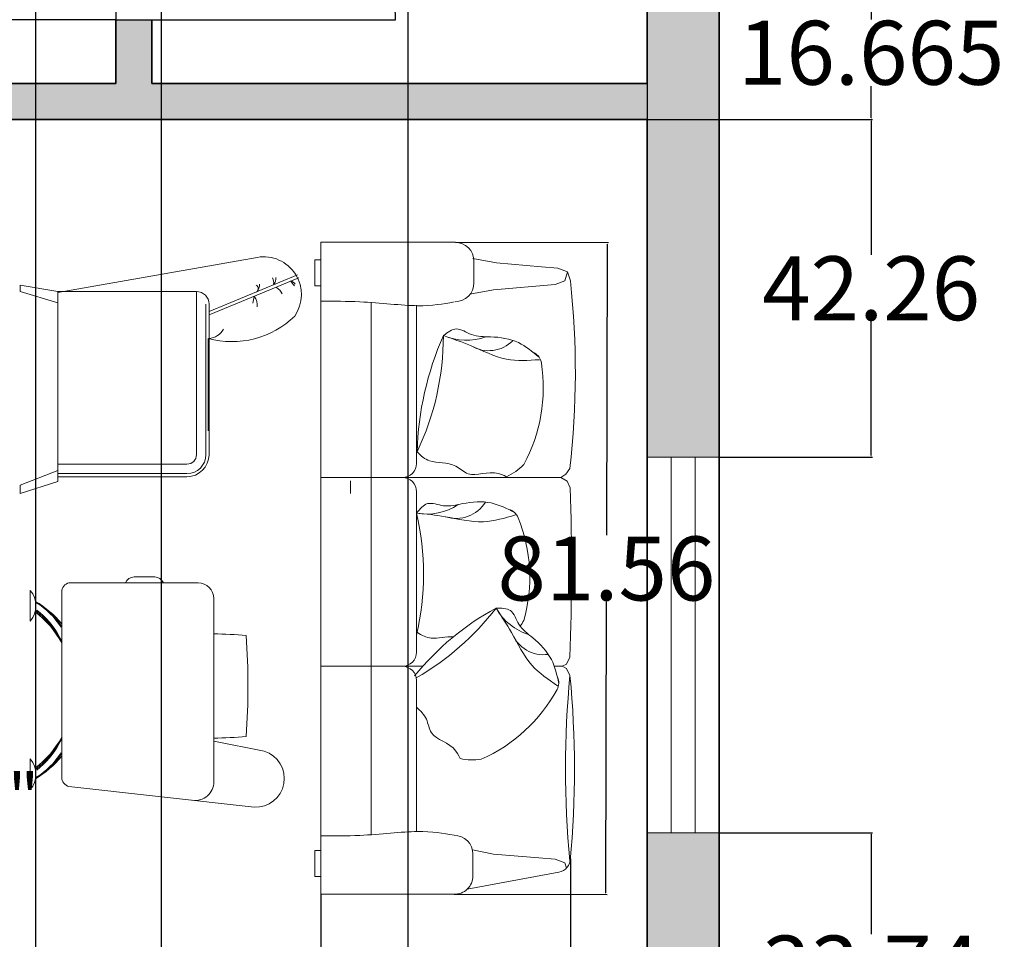
# Model space of a CAD drawing. Units: inches. Extents: x -24 to 368, y -370 to 58.
# Tile 6 of 9: x 235 to 358, y -255 to -140. Entities that reach past the tile are written whole.
import ezdxf

# ---------------------------------------------------------------- set-up
doc = ezdxf.new("R2010")
doc.units = ezdxf.units.IN
doc.header["$MEASUREMENT"] = 0
for name, color, linetype, lineweight in [('A-ANNO-DIMS', 2, 'Continuous', 18), ('A-AREA-IDEN', 7, 'Continuous', 18), ('A-WALL', 7, 'Continuous', 35), ('Furniture', 7, 'Continuous', 15)]:
    doc.layers.add(name, color=color, linetype=linetype, lineweight=lineweight)
for name, color, linetype, lineweight, true_color in [('A-DOOR', 40, 'Continuous', 25, 0xf8d731), ('A-GLAZ', 30, 'Continuous', 18, 0xf26722), ('A-WALL-PATT', 18, 'Continuous', 13, 0x000000)]:
    doc.layers.add(name, color=color, linetype=linetype, lineweight=lineweight, true_color=true_color)
doc.styles.get("Standard").update_dxf_attribs({"font": 'arial.ttf'})
doc.dimstyles.get("Standard").update_dxf_attribs({"dimtxt": 8, "dimasz": 0.18, "dimexe": 0.18, "dimexo": 0.0625, "dimgap": 0.09, "dimtad": 0, "dimtih": 1, "dimtoh": 1, "dimdec": 4, "dimzin": 0, "dimdsep": 46, "dimlunit": 3, "dimtxsty": 'Standard', "dimcen": 0.09, "dimclre": 5, "dimclrt": 6, "dimadec": 0, "dimazin": 0, "dimtfac": 1, "dimtdec": 4, "dimtofl": 0, "dimtmove": 0, "dimatfit": 3, "dimfxl": 1, "dimtolj": 1, "dimtzin": 0, "dimarcsym": 0})

# ---------------------------------------------------------------- blocks, each defined once
blk = doc.blocks.new('WINDOW-47-JAMB-DETAIL')
for p, q in [((0, 9), (47, 9)), ((0, 0), (0, 9)), ((0, 9), (0, 4.5)), ((47, 9), (47, 0)), ((0, 6), (47, 6)), ((0, 3), (47, 3)), ((47, 0), (0, 0))]:
    blk.add_line(p, q)
blk = doc.blocks.new('DOOR-SINGLE-35')
for p, q in [((0, 35), (0, 0)), ((0, 35), (4.5, 35)), ((0, 2), (35, 2)), ((0, 0), (35, 0)), ((0, 0), (4.5, 0))]:
    blk.add_line(p, q)
blk.add_arc((0, 0), 35, 0, 90)
blk = doc.blocks.new('*D34')
at = {"layer": 'A-ANNO-DIMS', "color": 5, "lineweight": -2, "transparency": 16777216}
for p, q in [((322.22, -241.61), (341.36, -241.61)), ((313.22, -275.36), (341.36, -275.36))]:
    blk.add_line(p, q, dxfattribs=at)
at = {"layer": 'A-ANNO-DIMS', "color": 0, "lineweight": -2, "transparency": 16777216}
for p, q in [((341.18, -241.79), (341.18, -254.31)), ((341.18, -275.18), (341.18, -262.66))]:
    blk.add_line(p, q, dxfattribs=at)
at = {"layer": 'A-ANNO-DIMS', "color": 0, "transparency": 16777216}
for points in [[(341.15, -241.79), (341.21, -241.79), (341.18, -241.61)], [(341.15, -275.18), (341.21, -275.18), (341.18, -275.36)]]:
    blk.add_solid(points, dxfattribs=at)
at = {"layer": 'Defpoints', "color": 0, "transparency": 16777216}
for p in [(322.16, -241.61), (341.18, -241.61), (313.16, -275.36)]:
    blk.add_point(p, dxfattribs=at)
at = {"layer": 'A-ANNO-DIMS', "color": 6, "transparency": 16777216, "insert": (341.18, -258.49), "char_height": 8, "attachment_point": 5}
blk.add_mtext('\\A1;33.74', dxfattribs=at)
blk = doc.blocks.new('*D35')
at = {"layer": 'A-ANNO-DIMS', "color": 5, "lineweight": -2, "transparency": 16777216}
for p, q in [((313.22, -152.36), (341.36, -152.36)), ((322.22, -194.61), (341.36, -194.61))]:
    blk.add_line(p, q, dxfattribs=at)
at = {"layer": 'A-ANNO-DIMS', "color": 0, "lineweight": -2, "transparency": 16777216}
for p, q in [((341.18, -152.54), (341.18, -169.31)), ((341.18, -194.43), (341.18, -177.66))]:
    blk.add_line(p, q, dxfattribs=at)
at = {"layer": 'A-ANNO-DIMS', "color": 0, "transparency": 16777216}
for points in [[(341.15, -152.54), (341.21, -152.54), (341.18, -152.36)], [(341.15, -194.43), (341.21, -194.43), (341.18, -194.61)]]:
    blk.add_solid(points, dxfattribs=at)
at = {"layer": 'Defpoints', "color": 0, "transparency": 16777216}
for p in [(313.16, -152.36), (341.18, -152.36), (322.16, -194.61)]:
    blk.add_point(p, dxfattribs=at)
at = {"layer": 'A-ANNO-DIMS', "color": 6, "transparency": 16777216, "insert": (341.18, -173.49), "char_height": 8, "attachment_point": 5}
blk.add_mtext('\\A1;42.26', dxfattribs=at)
blk = doc.blocks.new('*D36')
at = {"layer": 'A-ANNO-DIMS', "color": 5, "lineweight": -2, "transparency": 16777216}
for p, q in [((322.22, -135.69), (341.36, -135.69)), ((313.22, -152.36), (341.36, -152.36))]:
    blk.add_line(p, q, dxfattribs=at)
at = {"layer": 'A-ANNO-DIMS', "color": 0, "lineweight": -2, "transparency": 16777216}
for p, q in [((341.18, -135.87), (341.18, -139.85)), ((341.18, -152.18), (341.18, -148.2))]:
    blk.add_line(p, q, dxfattribs=at)
at = {"layer": 'A-ANNO-DIMS', "color": 0, "transparency": 16777216}
for points in [[(341.15, -135.87), (341.21, -135.87), (341.18, -135.69)], [(341.15, -152.18), (341.21, -152.18), (341.18, -152.36)]]:
    blk.add_solid(points, dxfattribs=at)
at = {"layer": 'Defpoints', "color": 0, "transparency": 16777216}
for p in [(322.16, -135.69), (341.18, -135.69), (313.16, -152.36)]:
    blk.add_point(p, dxfattribs=at)
at = {"layer": 'A-ANNO-DIMS', "color": 6, "transparency": 16777216, "insert": (341.18, -144.02), "char_height": 8, "attachment_point": 5}
blk.add_mtext('\\A1;16.665', dxfattribs=at)
blk = doc.blocks.new('*D43')
at = {"layer": 'A-ANNO-DIMS', "color": 5, "lineweight": -2, "transparency": 16777216}
for p, q in [((283.21, 24.58), (283.21, -363.55)), ((313.16, 24.58), (313.16, -363.55))]:
    blk.add_line(p, q, dxfattribs=at)
at = {"layer": 'A-ANNO-DIMS', "color": 0, "lineweight": -2, "transparency": 16777216}
for p, q in [((283.39, -363.37), (284.5, -363.37)), ((312.98, -363.37), (311.87, -363.37))]:
    blk.add_line(p, q, dxfattribs=at)
at = {"layer": 'A-ANNO-DIMS', "color": 0, "transparency": 16777216}
for points in [[(283.39, -363.34), (283.39, -363.4), (283.21, -363.37)], [(312.98, -363.34), (312.98, -363.4), (313.16, -363.37)]]:
    blk.add_solid(points, dxfattribs=at)
at = {"layer": 'Defpoints', "color": 0, "transparency": 16777216}
for p in [(283.21, 24.64), (313.16, 24.64), (313.16, -363.37)]:
    blk.add_point(p, dxfattribs=at)
at = {"layer": 'A-ANNO-DIMS', "color": 6, "transparency": 16777216, "insert": (298.19, -363.37), "char_height": 8, "attachment_point": 5}
blk.add_mtext('\\A1;29.95', dxfattribs=at)
blk = doc.blocks.new('*D59')
at = {"layer": 'A-ANNO-DIMS', "color": 5, "lineweight": -2, "transparency": 16777216}
for p, q in [((246.6, -139.91), (-15.03, -139.91)), ((246.6, -147.86), (-15.03, -147.86))]:
    blk.add_line(p, q, dxfattribs=at)
at = {"layer": 'A-ANNO-DIMS', "color": 0, "lineweight": -2, "transparency": 16777216}
for p, q in [((-14.85, -139.91), (-14.85, -139.73)), ((-14.85, -139.73), (-14.67, -139.73)), ((-14.85, -147.68), (-14.85, -140.09))]:
    blk.add_line(p, q, dxfattribs=at)
at = {"layer": 'A-ANNO-DIMS', "color": 0, "transparency": 16777216}
for points in [[(-14.88, -140.09), (-14.82, -140.09), (-14.85, -139.91)], [(-14.88, -147.68), (-14.82, -147.68), (-14.85, -147.86)]]:
    blk.add_solid(points, dxfattribs=at)
at = {"layer": 'Defpoints', "color": 0, "transparency": 16777216}
for p in [(-14.85, -139.91), (246.66, -139.91), (246.66, -147.86)]:
    blk.add_point(p, dxfattribs=at)
at = {"layer": 'A-ANNO-DIMS', "color": 6, "transparency": 16777216, "insert": (-4.2, -139.73), "char_height": 8, "attachment_point": 5}
blk.add_mtext('\\A1;7.95', dxfattribs=at)
blk = doc.blocks.new('*D61')
at = {"layer": 'A-ANNO-DIMS', "color": 5, "lineweight": -2, "transparency": 16777216}
for p, q in [((236.66, -275.29), (236.66, 52.85)), ((252.39, -275.29), (252.39, 52.85))]:
    blk.add_line(p, q, dxfattribs=at)
at = {"layer": 'A-ANNO-DIMS', "color": 0, "lineweight": -2, "transparency": 16777216}
for p, q in [((236.84, 52.67), (252.21, 52.67)), ((252.39, 52.67), (252.57, 52.67))]:
    blk.add_line(p, q, dxfattribs=at)
at = {"layer": 'A-ANNO-DIMS', "color": 0, "transparency": 16777216}
for points in [[(236.84, 52.7), (236.84, 52.64), (236.66, 52.67)], [(252.21, 52.7), (252.21, 52.64), (252.39, 52.67)]]:
    blk.add_solid(points, dxfattribs=at)
at = {"layer": 'Defpoints', "color": 0, "transparency": 16777216}
for p in [(252.39, 52.67), (236.66, -275.36), (252.39, -275.36)]:
    blk.add_point(p, dxfattribs=at)
at = {"layer": 'A-ANNO-DIMS', "color": 6, "transparency": 16777216, "insert": (265.78, 52.67), "char_height": 8, "attachment_point": 5}
blk.add_mtext('\\A1;15.73', dxfattribs=at)
blk = doc.blocks.new('*D66')
at = {"layer": 'A-ANNO-DIMS', "color": 5, "lineweight": -2, "transparency": 16777216}
for p, q in [((289.18, -167.74), (308.31, -167.77)), ((289.02, -249.3), (308.16, -249.33))]:
    blk.add_line(p, q, dxfattribs=at)
at = {"layer": 'A-ANNO-DIMS', "color": 0, "lineweight": -2, "transparency": 16777216}
for p, q in [((308.13, -167.95), (308.06, -204.38)), ((307.98, -249.15), (308.05, -212.73))]:
    blk.add_line(p, q, dxfattribs=at)
at = {"layer": 'A-ANNO-DIMS', "color": 0, "transparency": 16777216}
for points in [[(308.1, -167.95), (308.16, -167.95), (308.13, -167.77)], [(307.95, -249.15), (308.01, -249.15), (307.98, -249.33)]]:
    blk.add_solid(points, dxfattribs=at)
at = {"layer": 'Defpoints', "color": 0, "transparency": 16777216}
for p in [(289.11, -167.74), (288.96, -249.3), (307.98, -249.33)]:
    blk.add_point(p, dxfattribs=at)
at = {"layer": 'A-ANNO-DIMS', "color": 6, "transparency": 16777216, "insert": (308.05, -208.55), "char_height": 8, "attachment_point": 5}
blk.add_mtext('\\A1;81.56', dxfattribs=at)
blk = doc.blocks.new('*D67')
at = {"layer": 'A-ANNO-DIMS', "color": 5, "lineweight": -2, "transparency": 16777216}
for p, q in [((303.55, -244.87), (303.55, -363.55)), ((272.33, -249.36), (272.33, -363.55))]:
    blk.add_line(p, q, dxfattribs=at)
at = {"layer": 'A-ANNO-DIMS', "color": 0, "lineweight": -2, "transparency": 16777216}
for p, q in [((272.51, -363.37), (274.4, -363.37)), ((303.37, -363.37), (301.49, -363.37))]:
    blk.add_line(p, q, dxfattribs=at)
at = {"layer": 'A-ANNO-DIMS', "color": 0, "transparency": 16777216}
for points in [[(272.51, -363.34), (272.51, -363.4), (272.33, -363.37)], [(303.37, -363.34), (303.37, -363.4), (303.55, -363.37)]]:
    blk.add_solid(points, dxfattribs=at)
at = {"layer": 'Defpoints', "color": 0, "transparency": 16777216}
for p in [(303.55, -244.81), (272.33, -249.3), (303.55, -363.37)]:
    blk.add_point(p, dxfattribs=at)
at = {"layer": 'A-ANNO-DIMS', "color": 6, "transparency": 16777216, "insert": (287.94, -363.37), "char_height": 8, "attachment_point": 5}
blk.add_mtext('\\A1;31.22', dxfattribs=at)

msp = doc.modelspace()

# ---------------------------------------------------------------- hatches: boundary and pattern name
at = {"layer": 'A-WALL-PATT'}
h = msp.add_hatch(color=256, dxfattribs=at)
h.dxf.hatch_style = 1
h.paths.add_polyline_path([(13.1621, -93.8573), (80.4499, -93.8573), (80.4499, -89.3573), (13.1621, -89.3573), (13.1621, -61.0987), (4.1621, -61.0987), (4.1621, -149.8573), (13.1621, -149.8573)])
h.paths.add_polyline_path([(146.5668, -27.3573), (133.1621, -27.3573), (133.1621, 10.3323), (133.1272, 10.3313), (133.1621, 24.6427), (139.8141, 24.6427), (139.8141, 33.6427), (95.3329, 33.6427), (95.3329, 24.6427), (128.6621, 24.6427), (128.6621, -89.3573), (127.4499, -89.3573), (127.4499, -93.8573), (133.1621, -93.8573), (133.1621, -31.8573), (146.5668, -31.8573)])
h.paths.add_polyline_path([(197.6621, 24.6427), (236.2134, 24.6427), (236.2134, 33.6427), (169.8141, 33.6427), (169.8141, 24.6427), (193.1621, 24.6427), (193.1621, -27.3573), (181.5668, -27.3573), (181.5668, -31.8573), (193.1621, -31.8573), (193.1621, -95.8573), (199.2127, -95.8573), (199.2127, -91.3573), (197.6621, -91.3573)])
h.paths.add_polyline_path([(322.1621, -52.531), (313.1621, -52.531), (313.1621, -91.3573), (246.2127, -91.3573), (246.2127, -95.8573), (246.6621, -95.8573), (246.6621, -104.9077), (251.1621, -104.9077), (251.1621, -95.8573), (313.1621, -95.8573), (313.1621, -105.6922), (317.6621, -105.6922), (322.1621, -105.6922)])
h.paths.add_polyline_path([(322.1621, -135.6922), (313.1621, -135.6922), (313.1621, -147.8573), (251.1621, -147.8573), (251.1621, -139.9077), (246.6621, -139.9077), (246.6621, -147.8573), (199.43, -147.8573), (199.43, -152.3573), (313.1621, -152.3573), (313.1621, -194.6142), (317.6621, -194.6142), (322.1621, -194.6142)])
h.paths.add_polyline_path([(322.1621, -241.6142), (313.1621, -241.6142), (313.1621, -275.3573), (287.3912, -275.3573), (287.3912, -279.8573), (313.1621, -279.8573), (313.1621, -335.3573), (298.077, -335.3573), (298.077, -344.3573), (322.1621, -344.3573)])
h.paths.add_polyline_path([(263.077, -335.3573), (241.1621, -335.3573), (241.1621, -279.8573), (252.3912, -279.8573), (252.3912, -275.3573), (236.6621, -275.3573), (236.6621, -298.8573), (234.5689, -298.8573), (234.5689, -303.3573), (236.6621, -303.3573), (236.6621, -344.3573), (263.077, -344.3573), (263.077, -339.8573)])
h.paths.add_polyline_path([(175.5689, -298.8573), (131.6621, -298.8573), (131.6621, -152.3573), (164.43, -152.3573), (164.43, -147.8573), (127.1621, -147.8573), (127.1621, -232.8573), (117.1621, -232.8573), (117.1621, -237.3573), (127.1621, -237.3573), (127.1621, -335.3573), (84.4055, -335.3573), (84.4055, -344.3573), (131.6621, -344.3573), (131.6621, -303.3573), (175.5689, -303.3573)])
h.paths.add_polyline_path([(70.1621, -232.8573), (13.1621, -232.8573), (13.1621, -196.8573), (4.1621, -196.8573), (4.1621, -257.9061), (13.1621, -257.9061), (13.1621, -237.3573), (70.1621, -237.3573)])
h.paths.add_polyline_path([(13.1621, -304.9061), (4.1621, -304.9061), (4.1621, -344.3573), (37.4055, -344.3573), (37.4055, -335.3573), (13.1621, -335.3573)])
h.paths.add_polyline_path([(322.1621, 33.6427), (283.2134, 33.6427), (283.2134, 24.6427), (313.1621, 24.6427), (313.1621, 11.9273), (313.4656, 11.629), (313.1621, 11.629), (313.1621, -5.531), (322.1621, -5.531)])
h.paths.add_polyline_path([(48.3329, 33.6427), (4.1621, 33.6427), (4.1621, -14.0987), (13.1621, -14.0987), (13.1621, 24.6427), (48.3329, 24.6427)])

# ---------------------------------------------------------------- linework, layer by layer
at = {"layer": 'A-WALL'}
for p, q in [((322.1621, 33.6427), (322.1621, -344.3573)), ((313.1621, -95.8573), (313.1621, -147.8573)), ((246.6621, -139.9077), (246.6621, -147.8573)), ((251.1621, -139.9077), (251.1621, -147.8573)), ((199.43, -147.8573), (246.6621, -147.8573)), ((251.1621, -147.8573), (313.1621, -147.8573)), ((199.43, -152.3573), (313.1621, -152.3573)), ((313.1621, -152.3573), (313.1621, -232.8573)), ((313.1621, -232.8573), (313.1621, -275.3573))]:
    msp.add_line(p, q, dxfattribs=at)
at = {"layer": 'Furniture'}
for p, q in [((272.3319, -249.2987, 13.1343), (272.3323, -167.7325, -0.364)), ((289.1148, -167.7387, -0.364), (272.3323, -167.7325, -0.364)), ((264.3556, -169.6195), (239.4285, -174.032)), ((271.546, -169.9319), (271.546, -173.2035)), ((272.3323, -169.9319), (271.546, -169.9319)), ((291.3267, -169.7474, -0.364), (294.2813, -170.3225, -0.364)), ((291.4762, -170.1009, -0.364), (291.4762, -172.808, -0.364)), ((294.2813, -170.3225, -0.364), (299.9427, -170.8003, -0.364)), ((299.9427, -170.8003, -0.364), (301.9905, -170.9604, -0.364)), ((301.9905, -170.9604, -0.364), (303.1934, -171.4178, -0.364)), ((269.4035, -171.8269), (258.327, -176.3942)), ((269.5451, -172.1943), (258.327, -176.82)), ((302.8372, -172.5743, -0.364), (303.1934, -171.4178, -0.364)), ((303.1934, -171.4178, -0.364), (303.5496, -172.5743, -0.364)), ((234.705, -173.901), (234.705, -173.1136)), ((234.705, -173.1136), (239.4294, -173.901)), ((271.546, -173.2035), (272.3322, -173.2035, 0.5414)), ((290.9705, -174.2447, -0.364), (293.9251, -173.6696, -0.364)), ((293.9251, -173.6696, -0.364), (301.6343, -173.0317, -0.364)), ((301.6343, -173.0317, -0.364), (302.8372, -172.5743, -0.364)), ((239.4196, -175.2986), (234.705, -173.901)), ((239.4294, -173.901), (239.4196, -175.2986)), ((256.7522, -173.901), (239.4294, -173.901)), ((239.4294, -197.6823), (239.4294, -173.9994)), ((256.7522, -194.3143), (256.7522, -173.901)), ((257.9333, -179.7879), (257.9333, -175.4758)), ((258.327, -179.7879), (258.327, -175.4758)), ((278.5971, -175.267, 9.5261), (278.5971, -241.8677, 9.5261)), ((284.2893, -195.3958, -0.364), (284.2775, -175.6077, -0.0262)), ((257.9333, -194.3143), (257.9333, -179.7879)), ((258.2286, -179.7613), (258.2286, -191.308)), ((258.2286, -179.7613), (258.2286, -191.308)), ((258.327, -194.3143), (258.327, -179.7879)), ((239.4294, -195.4954), (255.5711, -195.4954)), ((234.705, -198.1234), (239.4294, -196.2877)), ((239.4294, -196.6765), (255.5711, -196.6765)), ((239.4294, -197.0702), (255.5711, -197.0702)), ((302.3533, -197.1751, -0.364), (302.9738, -196.7442, -0.364)), ((302.9738, -196.7442, -0.364), (303.4909, -196.0547, -0.364)), ((239.4294, -197.6823), (234.705, -199.1716)), ((234.705, -199.1716), (234.705, -198.1234)), ((272.3319, -197.1675, -0.364), (282.5177, -197.1675, -0.364)), ((276.0437, -197.5835), (276.0437, -199.1583)), ((277.9901, -197.1675, -0.364), (302.3643, -197.1675, -0.364)), ((302.3643, -197.1712, -0.364), (303.1207, -197.6059, -0.364)), ((303.1207, -197.6059, -0.364), (303.5305, -198.4697, -0.364)), ((284.2893, -219.0178, -0.364), (284.2893, -198.9391, -0.364)), ((256.9538, -210.3392), (240.8023, -210.3392)), ((251.5281, -209.6103), (248.9577, -209.6103)), ((235.9656, -211.2896), (235.9656, -215.1291)), ((239.9026, -211.4863), (239.9026, -234.6862)), ((258.9223, -235.2576), (258.9223, -212.3077)), ((302.5295, -220.7895, -0.364), (303.0772, -220.5042, -0.364)), ((303.0772, -220.5042, -0.364), (303.4909, -219.6423, -0.364)), ((282.5177, -220.7895, -0.364), (272.3319, -220.7895, -0.364)), ((285.0764, -220.7895, -0.364), (282.5177, -220.7895, -0.364)), ((302.5295, -220.7895, -0.364), (301.5279, -220.7895, -0.364)), ((302.5295, -220.7895, -0.364), (303.0772, -221.0748, -0.364)), ((303.0772, -221.0748, -0.364), (303.4929, -221.9407, -0.364)), ((284.2893, -241.4647, -0.364), (284.2893, -222.5611, -0.364)), ((265.2253, -231.4242), (258.9223, -230.1742)), ((235.9656, -236.2241), (235.9656, -232.3847)), ((263.9651, -238.4004), (240.8023, -235.8333)), ((271.546, -247.0993), (271.546, -243.8277)), ((271.546, -243.8277), (272.3322, -243.8277, 0.5414)), ((291.2845, -243.7734, -0.364), (293.9251, -244.2873, -0.364)), ((291.3326, -247.0106, -0.364), (291.3427, -244.3035, -0.364)), ((293.9251, -244.2873, -0.364), (299.5865, -244.7652, -0.364)), ((299.5865, -244.7652, -0.364), (301.6343, -244.9253, -0.364)), ((301.6343, -244.9253, -0.364), (302.8372, -245.3827, -0.364)), ((302.8372, -245.3827, -0.364), (303.0426, -246.0498, -0.364)), ((272.3323, -247.0993), (271.546, -247.0993)), ((290.6347, -248.6781, -0.364), (302.101, -246.551, -0.364)), ((272.3319, -249.2987, 13.1343), (288.9623, -249.2987, 13.1343))]:
    msp.add_line(p, q, dxfattribs=at)
for centre, radius, start, end in [((289.114, -170.1009, -0.364), 2.3622, 0, 89.981618), ((265.1615, -174.2763), 4.7261, 325.371325, 99.8192), ((265.4475, -172.7199), 0.9712, 344.422174, 32.142525), ((265.5414, -172.2758), 1.1464, 319.84282, 7.343635), ((263.9912, -173.5491), 0.5027, 299.967107, 60.032893), ((263.2451, -173.0449), 1.3973, 321.964512, 2.634632), ((265.8391, -174.9513), 1.8137, 24.431371, 59.771475), ((263.712, -176.7183), 6.3554, 33.590351, 40.720257), ((268.2286, -173.6106), 1.091, 35.267275, 72.137173), ((289.114, -172.808, -0.364), 2.3622, 270, 0), ((197.1179, -184.0487, -0.364), 107.0484, 353.560459, 6.153299), ((256.7522, -175.4758), 1.5748, 0, 90), ((256.91, -173.4302), 7.1466, 344.435682, 351.420044), ((262.5322, -175.6141), 1.8264, 353.208042, 37.731108), ((261.2023, -168.9398), 11.2227, 254.556461, 314.371536), ((258.056, -177.3878), 2.4153, 276.442908, 329.313492), ((322.6069, -194.9557, 13.1343), 38.2489, 156.033072, 178.468803), ((253.8716, -179.4037, 13.1343), 33.7842, 334.52723, 359.974645), ((290.4811, -172.7823, 13.1343), 7.2127, 246.938556, 290.230858), ((293.3222, -177.0329, 13.1343), 4.2668, 238.979624, 315.567993), ((298.165, -183.1186, 13.1343), 1.7716, 8.910642, 60.737084), ((280.1629, -185.9411, 13.1343), 19.9936, 331.316905, 8.910642), ((255.5711, -194.3143), 2.7559, 270, 0), ((255.5711, -194.3143), 2.3622, 270, 0), ((255.5711, -194.3143), 1.1811, 270, 0), ((282.5177, -195.3958, -0.364), 1.7716, 270, 0), ((292.9548, -191.1372, 13.1343), 6.4736, 293.698611, 317.179416), ((282.5177, -198.9391, -0.364), 1.7716, 0, 90), ((-11.4414, -208.4677, -0.364), 315.1305, 357.967837, 1.818093), ((285.5412, -194.5247, 13.1343), 7.2127, 260.004565, 303.296867), ((289.2696, -198.0229, 13.1343), 4.2668, 252.045633, 328.634002), ((251.3764, -209.2511, 13.1343), 33.7842, 346.959346, 13.040654), ((295.3629, -202.8563, 13.1343), 1.7716, 21.97665, 73.803093), ((278.465, -209.6755, 13.1343), 19.9936, 344.382914, 21.97665), ((241.0837, -211.4863), 1.1811, 103.782782, 180), ((248.9577, -210.7914), 1.1811, 90, 157.489764), ((251.5281, -210.7914), 1.1811, 22.510236, 90), ((256.9538, -212.3077), 1.9685, 0, 90), ((233.6985, -213.2094), 2.9707, 319.742467, 40.257533), ((230.384, -223.2785), 12.3111, 39.360519, 59.574967), ((231.7543, -221.2452), 9.8012, 34.372775, 60.150411), ((231.6873, -221.0337), 9.6127, 32.222968, 58.783777), ((228.8442, -224.0326), 12.672, 29.230031, 52.455872), ((229.8117, -223.0164), 11.4269, 27.983304, 53.52792), ((230.242, -222.1304), 10.6251, 28.420003, 52.110156), ((310.355, -243.203, 13.1343), 33.7842, 118.493386, 141.115548), ((267.4509, -192.9241, 13.1343), 33.7842, 299.834226, 322.456389), ((300.5206, -209.968, 13.1343), 7.2127, 209.4203, 252.712601), ((292.1004, -211.8451, 13.1343), 6.4736, 322.76952, 330.245425), ((258.855, -256.2559), 39.5187, 84.014312, 89.902501), ((300.1853, -215.0696, 13.1343), 4.2668, 201.461368, 278.049736), ((174.8754, -223.2579), 88.326, 355.906379, 4.093621), ((282.5177, -219.0178, -0.364), 1.7716, 270, 0), ((282.5177, -222.5611, -0.364), 1.7716, 0, 90), ((300.3201, -222.8459, 13.1343), 1.7716, 331.392385, 23.218828), ((426.077, -233.6789, -0.364), 123.1449, 174.530239, 185.336803), ((180.9087, -233.6789, -0.364), 123.1449, 354.663197, 5.469761), ((284.3227, -214.1211, 13.1343), 19.9936, 293.798648, 331.392385), ((228.8442, -223.4812), 12.672, 307.544128, 330.769969), ((229.8117, -224.4974), 11.4269, 306.47208, 332.016696), ((259.1106, -192.5935), 37.1712, 269.70971, 275.968983), ((231.6873, -226.4801), 9.6127, 301.216223, 327.777032), ((230.242, -225.3833), 10.6251, 307.889844, 331.579997), ((264.173, -234.8361), 3.5704, 266.660642, 72.859761), ((233.6985, -234.3044), 2.9707, 319.742467, 40.257533), ((230.384, -224.2353), 12.3111, 300.425033, 320.639481), ((231.7543, -226.2685), 9.8012, 299.849589, 325.627225), ((291.3042, -226.0328, 13.1343), 6.4736, 256.180354, 279.66116), ((241.0837, -234.6862), 1.1811, 180, 256.217218), ((256.5993, -235.2482), 2.323, 261.779114, 0.2322), ((288.9805, -244.2947, -0.364), 2.3622, 359.78593, 89.78593), ((301.7779, -244.8091, -0.364), 1.7716, 280.509138, 0), ((289.078, -247.0468, 13.1343), 2.2548, 267.058125, 0.920623)]:
    msp.add_arc(centre, radius, start, end, dxfattribs=at)
for points, knots in [([(288.9893, -175.2022, -0.364), (287.6226, -175.447, 1.8396), (284.7479, -175.962, 6.4746), (278.2328, -175.0947, 9.8816), (273.9547, -175.1144, 11.3657), (272.3319, -175.1218, 11.9286)], [0, 0, 0, 0, 7.67078163, 16.13451998, 21.30663444, 21.30663444, 21.30663444, 21.30663444]), ([(299.6194, -182.1069, 13.1343), (298.806, -181.4213, 13.1343), (297.0646, -179.9534, 13.1343), (293.9294, -179.4813, 13.1343), (291.2589, -179.6041, 13.1343), (289.3063, -178.124, 13.1343), (288.1874, -179.0016, 13.1343), (287.6558, -179.4187, 13.1343)], [0, 0, 0, 0, 3.13962122, 6.72122615, 9.13478433, 11.14737198, 12.96948872, 12.96948872, 12.96948872, 12.96948872]), ([(299.6683, -182.428, 13.1343), (298.2785, -182.516, 13.1343), (295.2528, -182.7076, 13.1343), (291.4437, -180.7044, 13.1343), (288.7897, -179.8035, 13.1343), (287.6558, -179.4187, 13.1343)], [0, 0, 0, 0, 4.1045126, 8.93575049, 12.53924172, 12.53924172, 12.53924172, 12.53924172]), ([(295.5567, -197.0649, 13.1343), (295.5567, -197.0649, 13.1343), (293.6204, -196.0066, 13.1343), (291.1812, -197.4776, 13.1343), (288.8005, -195.1002, 13.1343), (286.1669, -195.5204, 13.1343), (284.8463, -194.4961, 13.1343), (284.3716, -193.9337, 13.1343)], [27.78641734, 27.78641734, 27.78641734, 27.78641734, 60.3342139, 153.42843018, 198.91004811, 289.23861501, 341.46631935, 341.46631935, 341.46631935, 341.46631935]), ([(296.5509, -201.542, 13.1343), (295.6035, -201.058, 13.1343), (293.5754, -200.0218, 13.1343), (290.4147, -200.2706, 13.1343), (287.8411, -200.994, 13.1343), (285.6044, -199.9937, 13.1343), (284.7129, -201.1015, 13.1343), (284.2893, -201.628, 13.1343)], [0, 0, 0, 0, 3.13962122, 6.72122615, 9.13478433, 11.14737198, 12.96948872, 12.96948872, 12.96948872, 12.96948872]), ([(296.6712, -201.8437, 13.1343), (295.3372, -202.2436, 13.1343), (292.4332, -203.1143, 13.1343), (288.2698, -202.0241, 13.1343), (285.4808, -201.7465, 13.1343), (284.2893, -201.628, 13.1343)], [0, 0, 0, 0, 4.1045126, 8.93575049, 12.53924172, 12.53924172, 12.53924172, 12.53924172]), ([(302.0898, -222.9292, 13.1343), (301.8622, -221.89, 13.1343), (301.375, -219.6653, 13.1343), (299.1759, -217.3814, 13.1343), (296.9829, -215.8524, 13.1343), (296.3356, -213.4893, 13.1343), (294.9136, -213.504, 13.1343), (294.238, -213.511, 13.1343)], [0, 0, 0, 0, 3.13962122, 6.72122615, 9.13478433, 11.14737198, 12.96948872, 12.96948872, 12.96948872, 12.96948872]), ([(301.9331, -223.2137, 13.1343), (300.7772, -222.4371, 13.1343), (298.2606, -220.7464, 13.1343), (296.4594, -216.8377, 13.1343), (294.9029, -214.5068, 13.1343), (294.238, -213.511, 13.1343)], [0, 0, 0, 0, 4.1045126, 8.93575049, 12.53924172, 12.53924172, 12.53924172, 12.53924172]), ([(288.9091, -217.0985, 13.1343), (287.951, -217.0355, 13.1343), (286.3149, -217.5738, 13.1343), (284.9612, -216.9502, 13.1343), (284.3716, -216.5097, 13.1343)], [214.33234768, 214.33234768, 214.33234768, 214.33234768, 289.23861501, 341.46631935, 341.46631935, 341.46631935, 341.46631935]), ([(289.7579, -232.319, 13.1343), (289.7579, -232.319, 13.1343), (288.8666, -230.3004, 13.1343), (286.0361, -229.9816, 13.1343), (285.6711, -227.2175, 13.1343), (284.7607, -226.3468, 13.1343), (284.2893, -225.9038, 13.1343)], [27.78641734, 27.78641734, 27.78641734, 27.78641734, 60.3342139, 153.42843018, 198.91004811, 250.02765577, 250.02765577, 250.02765577, 250.02765577]), ([(288.9893, -241.9325, -0.364), (287.6226, -241.6876, 1.8396), (284.7479, -241.1726, 6.4746), (278.2328, -242.0399, 9.8816), (273.9547, -242.0203, 11.3657), (272.3319, -242.0128, 11.9286)], [0, 0, 0, 0, 7.67078163, 16.13451998, 21.30663444, 21.30663444, 21.30663444, 21.30663444])]:
    msp.add_open_spline(points, degree=3, knots=knots, dxfattribs=at)

# ---------------------------------------------------------------- block references
at = {"layer": 'A-DOOR'}
msp.add_blockref('DOOR-SINGLE-35', (246.662, -139.908), dxfattribs=at)
at = {"layer": 'A-GLAZ', "extrusion": (0, 0, -1), "zscale": -1, "rotation": 270.0000000000001}
msp.add_blockref('WINDOW-47-JAMB-DETAIL', (-322.1618, -194.6138), dxfattribs=at)

# ---------------------------------------------------------------- texts
at = {"layer": 'A-AREA-IDEN'}
msp.add_text('14\'5"X10\'10"', height=6, dxfattribs=at).set_placement((188.2434, -240.2094))

# ---------------------------------------------------------------- dimensions: what is measured, and where the dimension line sits
at = {"layer": 'A-ANNO-DIMS'}
for base, p1, p2, picture, middle in [((252.3912, 52.6658), (236.6621, -275.3573), (252.3912, -275.3573), '*D61', (265.7827, 52.6658)), ((313.1621, -363.3723), (283.2134, 24.6427), (313.1621, 24.6427), '*D43', (298.1877, -363.3723)), ((303.5496, -363.3723), (272.3319, -249.2987), (303.5496, -244.8091), '*D67', (287.9407, -363.3723))]:
    dim = msp.add_linear_dim(base=base, p1=p1, p2=p2, dimstyle='Standard', override={"dimdec": 2, "dimlfac": 1, "dimrnd": 0, "dimzin": 0, "dimdsep": 46, "dimlunit": 2}, dxfattribs=at)
    dim.commit()
    dim.dimension.update_dxf_attribs({"geometry": picture, "text_midpoint": middle})
for base, p1, p2, angle, override, picture, middle in [((-14.8529, -139.9077), (246.6621, -147.8573), (246.6621, -139.9077), 90, {"dimdec": 2, "dimlfac": 1, "dimrnd": 0, "dimzin": 0, "dimdsep": 46, "dimlunit": 2}, '*D59', (-4.1955, -139.7277)), ((341.1771, -135.6922), (313.1621, -152.3573), (322.1621, -135.6922), 90, {"dimdec": 3, "dimlfac": 1, "dimrnd": 0, "dimzin": 0, "dimdsep": 46, "dimlunit": 2}, '*D36', (341.1771, -144.0247)), ((341.1771, -152.3573), (322.1621, -194.6142), (313.1621, -152.3573), 90, {"dimdec": 2, "dimlfac": 1, "dimrnd": 0, "dimzin": 0, "dimdsep": 46, "dimlunit": 2}, '*D35', (341.1771, -173.4858)), ((307.9773, -249.3342), (289.1148, -167.7387), (288.9623, -249.2987), 269.892879, {"dimdec": 2, "dimlfac": 1, "dimrnd": 0, "dimzin": 0, "dimdsep": 46, "dimlunit": 2}, '*D66', (308.0535, -208.5542)), ((341.1771, -241.6142), (313.1621, -275.3573), (322.1621, -241.6142), 90, {"dimdec": 2, "dimlfac": 1, "dimrnd": 0, "dimzin": 0, "dimdsep": 46, "dimlunit": 2}, '*D34', (341.1771, -258.4858))]:
    dim = msp.add_linear_dim(base=base, p1=p1, p2=p2, angle=angle, dimstyle='Standard', override=override, dxfattribs=at)
    dim.commit()
    dim.dimension.update_dxf_attribs({"geometry": picture, "text_midpoint": middle})

doc.saveas('drawing.dxf')
